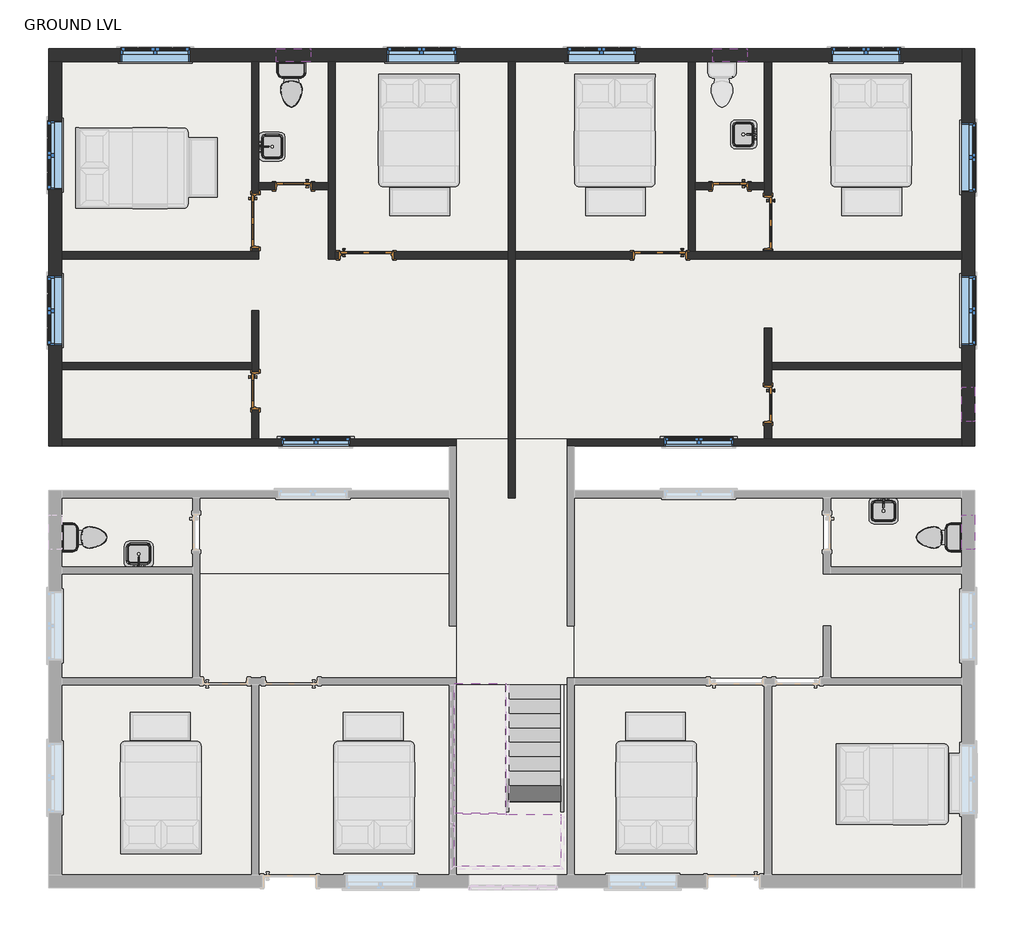
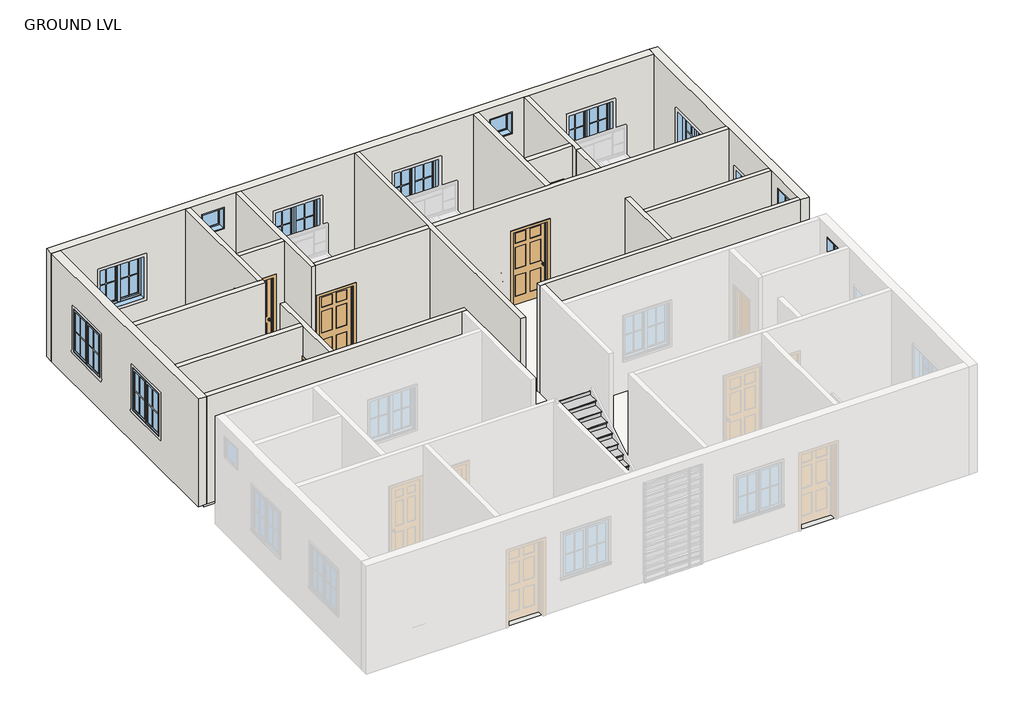
# One storey, part 3 of 4: 20 walls, 14 windows, 8 doors, 7 flow terminals, 7 slabs, 2 stair flights.
# Revit data of these elements (continued)
# Materials (continued)
#   "Steel, Polished": class "Metal", colour RGB 57 57 57, transparency 0, Description = "Polished steel", Cost = 0
#   "Laminate, Linen, Matte": class "Plastic", colour RGB 249 239 230, transparency 0, Description = "Plastic Laminate - Linen, Matte", Cost = 0
#   "marble flooring": class "Generic", colour RGB 120 120 120, transparency 0, Cost = 0
#   "wall paint": class "Generic", colour RGB 120 120 120, transparency 0, Cost = 0
#   "Glass": class "Glass", colour RGB 0 128 192, transparency 0.75, Description = "Soda Lime Glass", Cost = 0
#   "Sash": class "Wood", colour RGB 224 178 126, transparency 0, Cost = 0
#   "Wood - Stained": class "Wood", colour RGB 224 178 126, transparency 0, Cost = 0
#   "Clad - White": class "Wood", colour RGB 242 242 238, transparency 0, Cost = 0
